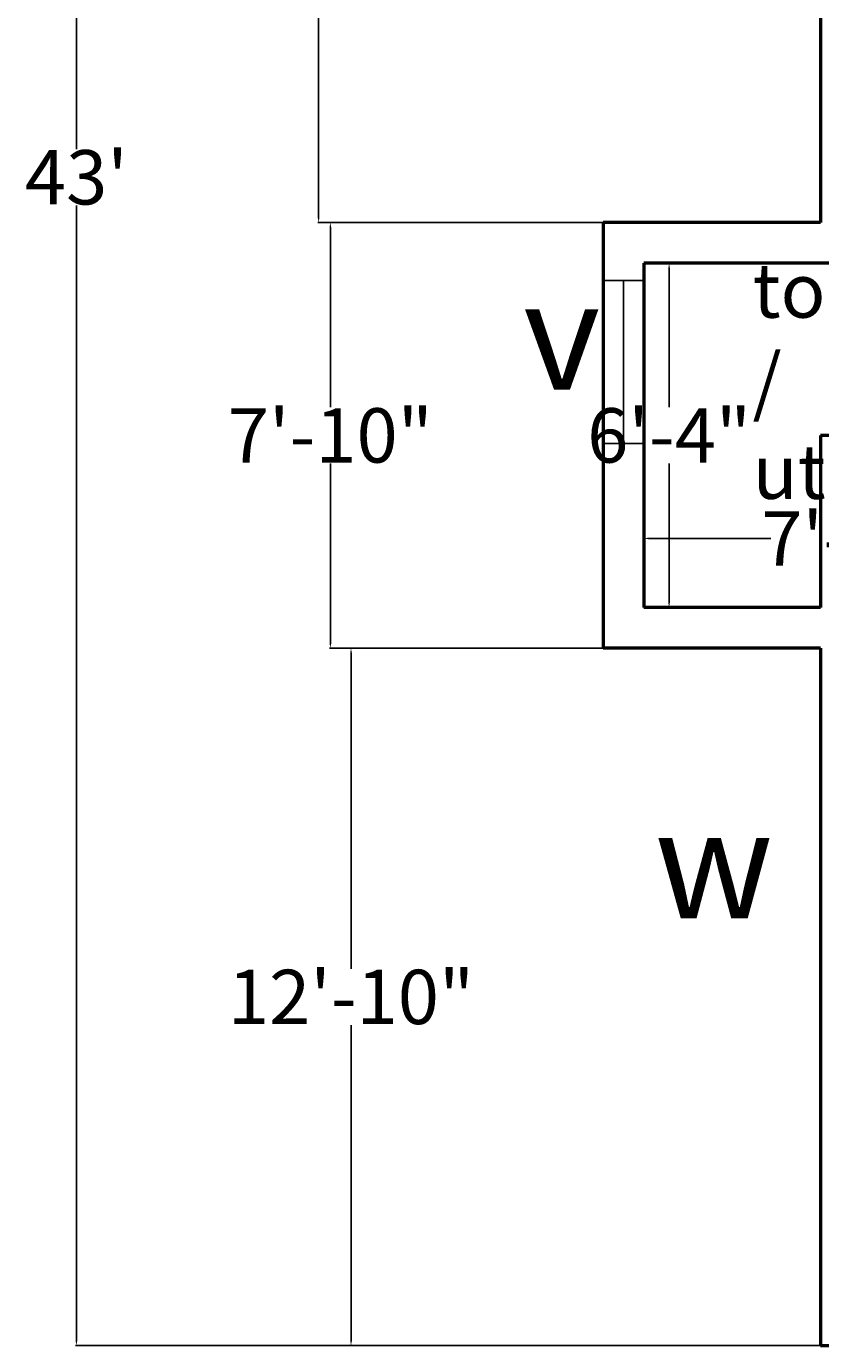
# Model space of a CAD drawing. Units: inches. Extents: x 409 to 7572, y 7 to 725.
# Tile 27 of 38: x 5502 to 5677, y 157 to 448. Entities that reach past the tile are written whole.
import ezdxf

# ---------------------------------------------------------------- set-up
doc = ezdxf.new("R2010")
doc.units = ezdxf.units.IN
doc.header["$MEASUREMENT"] = 0
for name, color, linetype, lineweight in [('A-ANNO-DIMS', 2, 'Continuous', 18), ('A-ANNO-SYMB', 3, 'Continuous', 25), ('A-AREA-IDEN', 7, 'Continuous', 25), ('A-GLAZ', 4, 'Continuous', 25), ('A-WALL', 7, 'Continuous', 50)]:
    doc.layers.add(name, color=color, linetype=linetype, lineweight=lineweight)
doc.styles.get("Standard").update_dxf_attribs({"font": 'arial.ttf'})
doc.dimstyles.get("Standard").update_dxf_attribs({"dimtxt": 2, "dimasz": 1, "dimexe": 0.18, "dimexo": 0.0625, "dimgap": 0.09, "dimtad": 0, "dimtih": 1, "dimtoh": 1, "dimdec": 0, "dimzin": 0, "dimdsep": 46, "dimlunit": 3, "dimtxsty": 'Standard', "dimcen": 0.09, "dimadec": 0, "dimazin": 0, "dimtfac": 1, "dimtdec": 0, "dimtofl": 0, "dimtmove": 0, "dimatfit": 3, "dimfxl": 1, "dimtolj": 1, "dimtzin": 0, "dimarcsym": 0})

# ---------------------------------------------------------------- blocks, each defined once
blk = doc.blocks.new('*D143')
at = {"layer": 'A-ANNO-DIMS', "color": 0, "lineweight": -2, "transparency": 16777216}
for p, q in [((5646.99, 395.53), (5643.17, 395.53)), ((5643.35, 394.53), (5643.35, 363.75)), ((5643.35, 320.53), (5643.35, 351.31)), ((5646.99, 319.53), (5643.17, 319.53))]:
    blk.add_line(p, q, dxfattribs=at)
at = {"layer": 'A-ANNO-DIMS', "color": 0, "transparency": 16777216}
for points in [[(5643.18, 394.53), (5643.51, 394.53), (5643.35, 395.53)], [(5643.18, 320.53), (5643.51, 320.53), (5643.35, 319.53)]]:
    blk.add_solid(points, dxfattribs=at)
at = {"layer": 'DEFPOINTS', "color": 0, "transparency": 16777216}
for p in [(5647.05, 395.53), (5643.35, 319.53), (5647.05, 319.53)]:
    blk.add_point(p, dxfattribs=at)
at = {"layer": 'A-ANNO-DIMS', "color": 0, "transparency": 16777216, "insert": (5643.35, 357.53), "char_height": 2, "attachment_point": 5}
blk.add_mtext('\\A1;{\\H6x;6\'-4"}', dxfattribs=at)
blk = doc.blocks.new('*D145')
at = {"layer": 'A-ANNO-DIMS', "color": 0, "lineweight": -2, "transparency": 16777216}
for p, q in [((5637.78, 346.33), (5637.78, 334.6)), ((5725.78, 346.33), (5725.78, 334.6)), ((5638.78, 334.78), (5665.79, 334.78)), ((5724.78, 334.78), (5697.77, 334.78))]:
    blk.add_line(p, q, dxfattribs=at)
at = {"layer": 'A-ANNO-DIMS', "color": 0, "transparency": 16777216}
for points in [[(5638.78, 334.95), (5638.78, 334.61), (5637.78, 334.78)], [(5724.78, 334.95), (5724.78, 334.61), (5725.78, 334.78)]]:
    blk.add_solid(points, dxfattribs=at)
at = {"layer": 'DEFPOINTS', "color": 0, "transparency": 16777216}
for p in [(5637.78, 346.39), (5725.78, 346.39), (5725.78, 334.78)]:
    blk.add_point(p, dxfattribs=at)
at = {"layer": 'A-ANNO-DIMS', "color": 0, "transparency": 16777216, "insert": (5681.78, 334.78), "char_height": 2, "attachment_point": 5}
blk.add_mtext('\\A1;{\\H6x;7\'-4"}', dxfattribs=at)
blk = doc.blocks.new('*D132')
at = {"layer": 'A-ANNO-DIMS', "color": 0, "lineweight": -2, "transparency": 16777216}
for p, q in [((5676.72, 672.53), (5565.82, 672.53)), ((5566, 671.53), (5566, 544.65)), ((5566, 405.53), (5566, 532.42)), ((5676.72, 404.53), (5565.82, 404.53))]:
    blk.add_line(p, q, dxfattribs=at)
at = {"layer": 'A-ANNO-DIMS', "color": 0, "transparency": 16777216}
for points in [[(5565.84, 671.53), (5566.17, 671.53), (5566, 672.53)], [(5565.84, 405.53), (5566.17, 405.53), (5566, 404.53)]]:
    blk.add_solid(points, dxfattribs=at)
at = {"layer": 'DEFPOINTS', "color": 0, "transparency": 16777216}
for p in [(5676.78, 672.53), (5566, 404.53), (5676.78, 404.53)]:
    blk.add_point(p, dxfattribs=at)
at = {"layer": 'A-ANNO-DIMS', "color": 0, "transparency": 16777216, "insert": (5566, 538.53), "char_height": 2, "attachment_point": 5}
blk.add_mtext('\\A1;{\\H6x;22\'-4"}', dxfattribs=at)
blk = doc.blocks.new('*D133')
at = {"layer": 'A-ANNO-DIMS', "color": 0, "lineweight": -2, "transparency": 16777216}
for p, q in [((5628.72, 404.53), (5568.41, 404.53)), ((5568.59, 403.53), (5568.59, 363.75)), ((5568.59, 311.53), (5568.59, 351.31)), ((5628.72, 310.53), (5568.41, 310.53))]:
    blk.add_line(p, q, dxfattribs=at)
at = {"layer": 'A-ANNO-DIMS', "color": 0, "transparency": 16777216}
for points in [[(5568.43, 403.53), (5568.76, 403.53), (5568.59, 404.53)], [(5568.43, 311.53), (5568.76, 311.53), (5568.59, 310.53)]]:
    blk.add_solid(points, dxfattribs=at)
at = {"layer": 'DEFPOINTS', "color": 0, "transparency": 16777216}
for p in [(5628.78, 404.53), (5568.59, 310.53), (5628.78, 310.53)]:
    blk.add_point(p, dxfattribs=at)
at = {"layer": 'A-ANNO-DIMS', "color": 0, "transparency": 16777216, "insert": (5568.59, 357.53), "char_height": 2, "attachment_point": 5}
blk.add_mtext('\\A1;{\\H6x;7\'-10"}', dxfattribs=at)
blk = doc.blocks.new('*D134')
at = {"layer": 'A-ANNO-DIMS', "color": 0, "lineweight": -2, "transparency": 16777216}
for p, q in [((5676.72, 310.53), (5572.97, 310.53)), ((5573.15, 309.53), (5573.15, 239.75)), ((5573.15, 157.53), (5573.15, 227.31)), ((5676.72, 156.53), (5572.97, 156.53))]:
    blk.add_line(p, q, dxfattribs=at)
at = {"layer": 'A-ANNO-DIMS', "color": 0, "transparency": 16777216}
for points in [[(5572.99, 309.53), (5573.32, 309.53), (5573.15, 310.53)], [(5572.99, 157.53), (5573.32, 157.53), (5573.15, 156.53)]]:
    blk.add_solid(points, dxfattribs=at)
at = {"layer": 'DEFPOINTS', "color": 0, "transparency": 16777216}
for p in [(5676.78, 310.53), (5573.15, 156.53), (5676.78, 156.53)]:
    blk.add_point(p, dxfattribs=at)
at = {"layer": 'A-ANNO-DIMS', "color": 0, "transparency": 16777216, "insert": (5573.15, 233.53), "char_height": 2, "attachment_point": 5}
blk.add_mtext('\\A1;{\\H6x;12\'-10"}', dxfattribs=at)
blk = doc.blocks.new('*D121')
at = {"layer": 'A-ANNO-DIMS', "color": 0, "lineweight": -2, "transparency": 16777216}
for p, q in [((5676.72, 672.53), (5512.37, 672.53)), ((5512.55, 671.53), (5512.55, 420.75)), ((5512.55, 157.53), (5512.55, 408.31)), ((5676.72, 156.53), (5512.37, 156.53))]:
    blk.add_line(p, q, dxfattribs=at)
at = {"layer": 'A-ANNO-DIMS', "color": 0, "transparency": 16777216}
for points in [[(5512.38, 671.53), (5512.71, 671.53), (5512.55, 672.53)], [(5512.38, 157.53), (5512.71, 157.53), (5512.55, 156.53)]]:
    blk.add_solid(points, dxfattribs=at)
at = {"layer": 'DEFPOINTS', "color": 0, "transparency": 16777216}
for p in [(5676.78, 672.53), (5512.55, 156.53), (5676.78, 156.53)]:
    blk.add_point(p, dxfattribs=at)
at = {"layer": 'A-ANNO-DIMS', "color": 0, "transparency": 16777216, "insert": (5512.55, 414.53), "char_height": 2, "attachment_point": 5}
blk.add_mtext("\\A1;{\\H6x;43'}", dxfattribs=at)
blk = doc.blocks.new('VENT-36')
blk.add_line((5633.28, 355.73), (5633.28, 391.73))
blk.add_lwpolyline([(5628.78, 355.73), (5628.78, 391.73), (5637.78, 391.73), (5637.78, 355.73)], close=True)

msp = doc.modelspace()

# ---------------------------------------------------------------- linework, layer by layer
at = {"layer": 'A-WALL'}
for p, q in [((5676.78, 672.53), (5676.78, 404.53)), ((5676.78, 404.53), (5628.78, 404.53)), ((5628.78, 404.53), (5628.78, 310.53)), ((5685.78, 395.53), (5637.78, 395.53)), ((5637.78, 395.53), (5637.78, 319.53)), ((5676.78, 357.53), (5676.78, 319.53)), ((5685.78, 357.53), (5676.78, 357.53)), ((5676.78, 319.53), (5637.78, 319.53)), ((5676.78, 310.53), (5628.78, 310.53)), ((5676.78, 310.53), (5676.78, 156.53)), ((5676.78, 156.53), (6050.78, 156.53))]:
    msp.add_line(p, q, dxfattribs=at)

# ---------------------------------------------------------------- block references
at = {"layer": 'A-GLAZ'}
msp.add_blockref('VENT-36', (0, 0), dxfattribs=at)

# ---------------------------------------------------------------- texts
at = {"layer": 'A-ANNO-SYMB', "char_height": 24, "attachment_point": 1}
for s, insert in [('v', (5611.12, 391.62)), ('w', (5640.1, 274.86))]:
    msp.add_mtext_dynamic_manual_height_columns(s, width=18.2582, gutter_width=1, heights=[0], dxfattribs=dict(at, insert=insert))
at = {"layer": 'A-AREA-IDEN', "insert": (5661.78, 395.53), "char_height": 12, "attachment_point": 1}
msp.add_mtext_dynamic_manual_height_columns('toilet / utility', width=49.2946, gutter_width=1, heights=[0], dxfattribs=at)

# ---------------------------------------------------------------- dimensions: what is measured, and where the dimension line sits
at = {"layer": 'A-ANNO-DIMS'}
for base, p1, p2, picture, middle in [((5512.55, 156.53), (5676.78, 672.53), (5676.78, 156.53), '*D121', (5512.55, 414.53)), ((5566, 404.53), (5676.78, 672.53), (5676.78, 404.53), '*D132', (5566, 538.53)), ((5568.59, 310.53), (5628.78, 404.53), (5628.78, 310.53), '*D133', (5568.59, 357.53)), ((5643.35, 319.53), (5647.05, 395.53), (5647.05, 319.53), '*D143', (5643.35, 357.53)), ((5573.15, 156.53), (5676.78, 310.53), (5676.78, 156.53), '*D134', (5573.15, 233.53))]:
    dim = msp.add_linear_dim(base=base, p1=p1, p2=p2, angle=90, text='{\\H6x;<>}', dimstyle='Standard', override={"dimclrd": 0, "dimclre": 0, "dimclrt": 0}, dxfattribs=at)
    dim.commit()
    dim.dimension.update_dxf_attribs({"geometry": picture, "text_midpoint": middle})
dim = msp.add_linear_dim(base=(5725.78, 334.78), p1=(5637.78, 346.39), p2=(5725.78, 346.39), text='{\\H6x;<>}', dimstyle='Standard', override={"dimclrd": 0, "dimclre": 0, "dimclrt": 0}, dxfattribs=at)
dim.commit()
dim.dimension.update_dxf_attribs({"geometry": '*D145', "text_midpoint": (5681.78, 334.78)})

doc.saveas('drawing.dxf')
